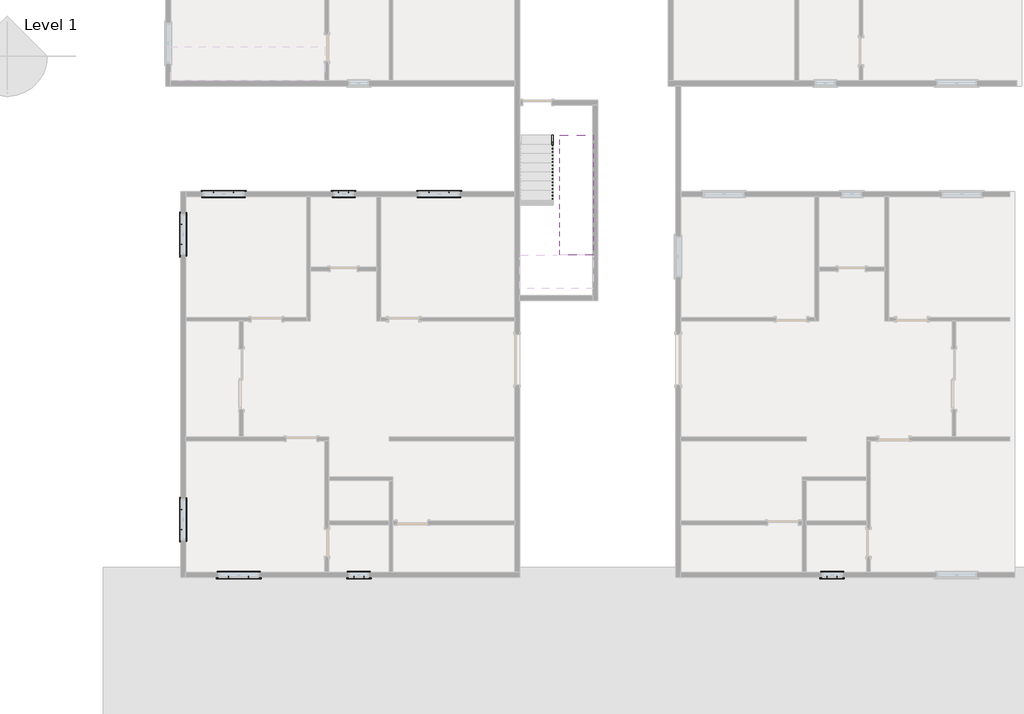
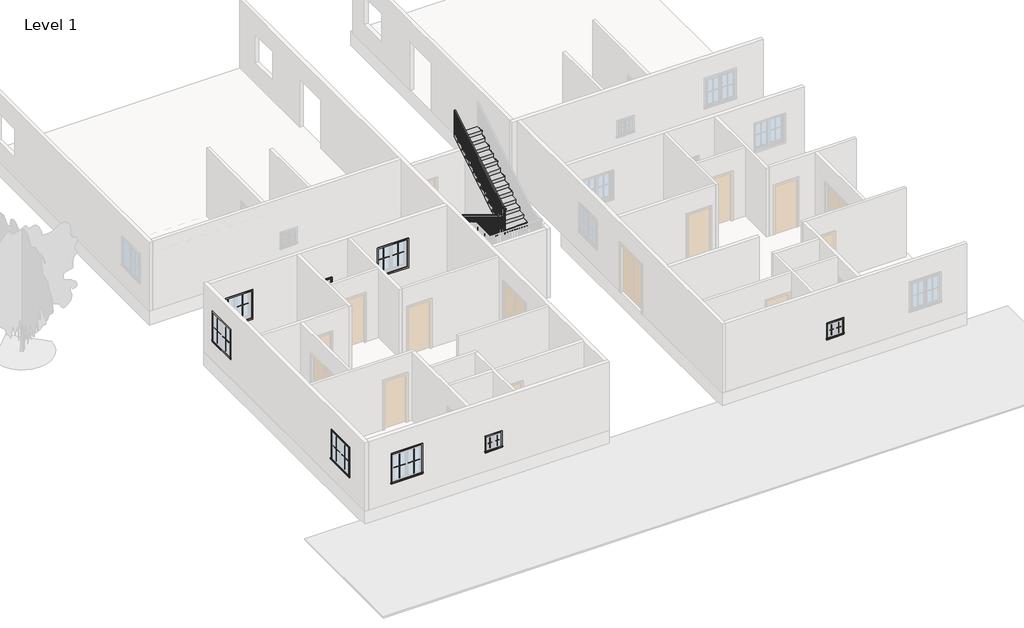
# One storey, part 5 of 7: 32 proxies, 1 railing, 1 stair flight.
"""IFC4 building model written with IfcOpenShell, lengths in millimetres."""

from ifc_helpers import new_model, si_unit, frame, origin, place, context, project, spatial, polyline, outline, extrude, faceted_brep, transform, mapped, element, save
from components import muntin_pattern_2x2_muntin_pattern_2x2_4dfeb3f3, muntin_pattern_2x2_muntin_pattern_2x2_e852a7e4, muntin_pattern_2x2_muntin_pattern_2x2_0961b91c, muntin_pattern_2x2_muntin_pattern_2x2_cae9449b, trim_window_exterior_flat_with_sill_7cfdd449, trim_window_exterior_flat_with_sill_858dc10d, trim_window_interior_flat_picture_frame_f1e0b15b, trim_window_interior_flat_picture_frame_3927330c

model = new_model("IFC4")

# Units and contexts
model_context = context("Model", 3, world=origin())
ifc_project = project(units=[si_unit("LENGTHUNIT", "METRE", prefix="MILLI")], contexts=[model_context])

# Site, building, storey
site = spatial("IfcSite", under=ifc_project)
building = spatial("IfcBuilding", under=site)
storey = spatial("IfcBuildingStorey", under=building, Name="Level 1", Elevation=0.0)

# Proxies
placement = place(None, origin())
muntin_pattern_2x2_muntin_pattern_2x2_shape = muntin_pattern_2x2_muntin_pattern_2x2_4dfeb3f3(model_context)
element("IfcBuildingElementProxy", 1, Name="Muntin Pattern_2x2 : Muntin Pattern_2x2", ObjectType="Muntin Pattern_2x2 : Muntin Pattern_2x2", at=placement, inside=storey, context=model_context, shape_type="MappedRepresentation", body=[
    mapped(muntin_pattern_2x2_muntin_pattern_2x2_shape, transform((-12764.9599256, -1071.5314015, 984.25), x_axis=(1.0, 0.0, 0.0), y_axis=(0.0, 1.0, 0.0), z_axis=(0.0, 0.0, 1.0))),
])
element("IfcBuildingElementProxy", 2, Name="Muntin Pattern_2x2 : Muntin Pattern_2x2", ObjectType="Muntin Pattern_2x2 : Muntin Pattern_2x2", at=placement, inside=storey, context=model_context, shape_type="MappedRepresentation", body=[
    mapped(muntin_pattern_2x2_muntin_pattern_2x2_shape, transform((-13747.0413899, -2660.6442701, 984.25), x_axis=(0.0, 1.0, 0.0), y_axis=(-1.0, 0.0, 0.0), z_axis=(0.0, 0.0, 1.0))),
])
element("IfcBuildingElementProxy", 3, Name="Muntin Pattern_2x2 : Muntin Pattern_2x2", ObjectType="Muntin Pattern_2x2 : Muntin Pattern_2x2", at=placement, inside=storey, context=model_context, shape_type="MappedRepresentation", body=[
    mapped(muntin_pattern_2x2_muntin_pattern_2x2_shape, transform((-6243.5099256, -1071.5314015, 984.25), x_axis=(1.0, 0.0, 0.0), y_axis=(0.0, 1.0, 0.0), z_axis=(0.0, 0.0, 1.0))),
])
element("IfcBuildingElementProxy", 4, Name="Muntin Pattern_2x2 : Muntin Pattern_2x2", ObjectType="Muntin Pattern_2x2 : Muntin Pattern_2x2", at=placement, inside=storey, context=model_context, shape_type="MappedRepresentation", body=[
    mapped(muntin_pattern_2x2_muntin_pattern_2x2_shape, transform((-13747.0413899, -11296.6442701, 984.25), x_axis=(0.0, 1.0, 0.0), y_axis=(-1.0, 0.0, 0.0), z_axis=(0.0, 0.0, 1.0))),
])
element("IfcBuildingElementProxy", 5, Name="Muntin Pattern_2x2 : Muntin Pattern_2x2", ObjectType="Muntin Pattern_2x2 : Muntin Pattern_2x2", at=placement, inside=storey, context=model_context, shape_type="MappedRepresentation", body=[
    mapped(muntin_pattern_2x2_muntin_pattern_2x2_shape, transform((-11701.3349256, -12736.4814015, 984.25), x_axis=(-1.0, 0.0, 0.0), y_axis=(0.0, -1.0, 0.0), z_axis=(0.0, 0.0, 1.0))),
])
muntin_pattern_2x2_muntin_pattern_2x2_2_shape = muntin_pattern_2x2_muntin_pattern_2x2_e852a7e4(model_context)
element("IfcBuildingElementProxy", 6, Name="Muntin Pattern_2x2 : Muntin Pattern_2x2", ObjectType="Muntin Pattern_2x2 : Muntin Pattern_2x2", at=placement, inside=storey, context=model_context, shape_type="MappedRepresentation", body=[
    mapped(muntin_pattern_2x2_muntin_pattern_2x2_2_shape, transform((-12158.5349256, -1071.5314015, 984.25), x_axis=(-1.0, 0.0, 0.0), y_axis=(0.0, -1.0, 0.0), z_axis=(0.0, 0.0, 1.0))),
])
element("IfcBuildingElementProxy", 7, Name="Muntin Pattern_2x2 : Muntin Pattern_2x2", ObjectType="Muntin Pattern_2x2 : Muntin Pattern_2x2", at=placement, inside=storey, context=model_context, shape_type="MappedRepresentation", body=[
    mapped(muntin_pattern_2x2_muntin_pattern_2x2_2_shape, transform((-13747.0413899, -2054.2192701, 984.25), x_axis=(0.0, -1.0, 0.0), y_axis=(1.0, 0.0, 0.0), z_axis=(0.0, 0.0, 1.0))),
])
element("IfcBuildingElementProxy", 8, Name="Muntin Pattern_2x2 : Muntin Pattern_2x2", ObjectType="Muntin Pattern_2x2 : Muntin Pattern_2x2", at=placement, inside=storey, context=model_context, shape_type="MappedRepresentation", body=[
    mapped(muntin_pattern_2x2_muntin_pattern_2x2_2_shape, transform((-5637.0849256, -1071.5314015, 984.25), x_axis=(-1.0, 0.0, 0.0), y_axis=(0.0, -1.0, 0.0), z_axis=(0.0, 0.0, 1.0))),
])
element("IfcBuildingElementProxy", 9, Name="Muntin Pattern_2x2 : Muntin Pattern_2x2", ObjectType="Muntin Pattern_2x2 : Muntin Pattern_2x2", at=placement, inside=storey, context=model_context, shape_type="MappedRepresentation", body=[
    mapped(muntin_pattern_2x2_muntin_pattern_2x2_2_shape, transform((-13747.0413899, -10690.2192701, 984.25), x_axis=(0.0, -1.0, 0.0), y_axis=(1.0, 0.0, 0.0), z_axis=(0.0, 0.0, 1.0))),
])
element("IfcBuildingElementProxy", 10, Name="Muntin Pattern_2x2 : Muntin Pattern_2x2", ObjectType="Muntin Pattern_2x2 : Muntin Pattern_2x2", at=placement, inside=storey, context=model_context, shape_type="MappedRepresentation", body=[
    mapped(muntin_pattern_2x2_muntin_pattern_2x2_2_shape, transform((-12307.7599256, -12736.4814015, 984.25), x_axis=(1.0, 0.0, 0.0), y_axis=(0.0, 1.0, 0.0), z_axis=(0.0, 0.0, 1.0))),
])
muntin_pattern_2x2_muntin_pattern_2x2_3_shape = muntin_pattern_2x2_muntin_pattern_2x2_0961b91c(model_context)
element("IfcBuildingElementProxy", 11, Name="Muntin Pattern_2x2 : Muntin Pattern_2x2", ObjectType="Muntin Pattern_2x2 : Muntin Pattern_2x2", at=placement, inside=storey, context=model_context, shape_type="MappedRepresentation", body=[
    mapped(muntin_pattern_2x2_muntin_pattern_2x2_3_shape, transform((-8980.3599256, -1071.5314015, 984.25), x_axis=(1.0, 0.0, 0.0), y_axis=(0.0, 1.0, 0.0), z_axis=(0.0, 0.0, 1.0))),
])
element("IfcBuildingElementProxy", 12, Name="Muntin Pattern_2x2 : Muntin Pattern_2x2", ObjectType="Muntin Pattern_2x2 : Muntin Pattern_2x2", at=placement, inside=storey, context=model_context, shape_type="MappedRepresentation", body=[
    mapped(muntin_pattern_2x2_muntin_pattern_2x2_3_shape, transform((-8216.4719485, -12736.4814015, 984.25), x_axis=(-1.0, 0.0, 0.0), y_axis=(0.0, -1.0, 0.0), z_axis=(0.0, 0.0, 1.0))),
])
element("IfcBuildingElementProxy", 13, Name="Muntin Pattern_2x2 : Muntin Pattern_2x2", ObjectType="Muntin Pattern_2x2 : Muntin Pattern_2x2", at=placement, inside=storey, context=model_context, shape_type="MappedRepresentation", body=[
    mapped(muntin_pattern_2x2_muntin_pattern_2x2_3_shape, transform((6102.7780515, -12736.4814015, 984.25), x_axis=(-1.0, 0.0, 0.0), y_axis=(0.0, -1.0, 0.0), z_axis=(0.0, 0.0, 1.0))),
])
muntin_pattern_2x2_muntin_pattern_2x2_4_shape = muntin_pattern_2x2_muntin_pattern_2x2_cae9449b(model_context)
element("IfcBuildingElementProxy", 14, Name="Muntin Pattern_2x2 : Muntin Pattern_2x2", ObjectType="Muntin Pattern_2x2 : Muntin Pattern_2x2", at=placement, inside=storey, context=model_context, shape_type="MappedRepresentation", body=[
    mapped(muntin_pattern_2x2_muntin_pattern_2x2_4_shape, transform((-8678.7349256, -1071.5314015, 984.25), x_axis=(-1.0, 0.0, 0.0), y_axis=(0.0, -1.0, 0.0), z_axis=(0.0, 0.0, 1.0))),
])
element("IfcBuildingElementProxy", 15, Name="Muntin Pattern_2x2 : Muntin Pattern_2x2", ObjectType="Muntin Pattern_2x2 : Muntin Pattern_2x2", at=placement, inside=storey, context=model_context, shape_type="MappedRepresentation", body=[
    mapped(muntin_pattern_2x2_muntin_pattern_2x2_4_shape, transform((-8518.0969485, -12736.4814015, 984.25), x_axis=(1.0, 0.0, 0.0), y_axis=(0.0, 1.0, 0.0), z_axis=(0.0, 0.0, 1.0))),
])
element("IfcBuildingElementProxy", 16, Name="Muntin Pattern_2x2 : Muntin Pattern_2x2", ObjectType="Muntin Pattern_2x2 : Muntin Pattern_2x2", at=placement, inside=storey, context=model_context, shape_type="MappedRepresentation", body=[
    mapped(muntin_pattern_2x2_muntin_pattern_2x2_4_shape, transform((5801.1530515, -12736.4814015, 984.25), x_axis=(1.0, 0.0, 0.0), y_axis=(0.0, 1.0, 0.0), z_axis=(0.0, 0.0, 1.0))),
])
trim_window_exterior_flat_with_sill_shape = trim_window_exterior_flat_with_sill_7cfdd449(model_context)
element("IfcBuildingElementProxy", 17, Name="Trim-Window-Exterior-Flat : with Sill", ObjectType="Trim-Window-Exterior-Flat : with Sill", at=placement, inside=storey, context=model_context, shape_type="MappedRepresentation", body=[
    mapped(trim_window_exterior_flat_with_sill_shape, transform((-12461.7474256, -1062.0064015, 2133.6), x_axis=(-1.0, 0.0, 0.0), y_axis=(0.0, 0.0, 1.0), z_axis=(0.0, 1.0, 0.0))),
])
element("IfcBuildingElementProxy", 18, Name="Trim-Window-Exterior-Flat : with Sill", ObjectType="Trim-Window-Exterior-Flat : with Sill", at=placement, inside=storey, context=model_context, shape_type="MappedRepresentation", body=[
    mapped(trim_window_exterior_flat_with_sill_shape, transform((-13756.5663899, -2357.4317701, 2133.6), x_axis=(0.0, -1.0, 0.0), y_axis=(0.0, 0.0, 1.0), z_axis=(-1.0, 0.0, 0.0))),
])
element("IfcBuildingElementProxy", 19, Name="Trim-Window-Exterior-Flat : with Sill", ObjectType="Trim-Window-Exterior-Flat : with Sill", at=placement, inside=storey, context=model_context, shape_type="MappedRepresentation", body=[
    mapped(trim_window_exterior_flat_with_sill_shape, transform((-5940.2974256, -1062.0064015, 2133.6), x_axis=(-1.0, 0.0, 0.0), y_axis=(0.0, 0.0, 1.0), z_axis=(0.0, 1.0, 0.0))),
])
element("IfcBuildingElementProxy", 20, Name="Trim-Window-Exterior-Flat : with Sill", ObjectType="Trim-Window-Exterior-Flat : with Sill", at=placement, inside=storey, context=model_context, shape_type="MappedRepresentation", body=[
    mapped(trim_window_exterior_flat_with_sill_shape, transform((-13756.5663899, -10993.4317701, 2133.6), x_axis=(0.0, -1.0, 0.0), y_axis=(0.0, 0.0, 1.0), z_axis=(-1.0, 0.0, 0.0))),
])
element("IfcBuildingElementProxy", 21, Name="Trim-Window-Exterior-Flat : with Sill", ObjectType="Trim-Window-Exterior-Flat : with Sill", at=placement, inside=storey, context=model_context, shape_type="MappedRepresentation", body=[
    mapped(trim_window_exterior_flat_with_sill_shape, transform((-12004.5474256, -12746.0064015, 2133.6), x_axis=(1.0, 0.0, 0.0), y_axis=(0.0, 0.0, 1.0), z_axis=(0.0, -1.0, 0.0))),
])
trim_window_exterior_flat_with_sill_2_shape = trim_window_exterior_flat_with_sill_858dc10d(model_context)
element("IfcBuildingElementProxy", 22, Name="Trim-Window-Exterior-Flat : with Sill", ObjectType="Trim-Window-Exterior-Flat : with Sill", at=placement, inside=storey, context=model_context, shape_type="MappedRepresentation", body=[
    mapped(trim_window_exterior_flat_with_sill_2_shape, transform((-8829.5474256, -1062.0064015, 1524.0), x_axis=(-1.0, 0.0, 0.0), y_axis=(0.0, 0.0, 1.0), z_axis=(0.0, 1.0, 0.0))),
])
element("IfcBuildingElementProxy", 23, Name="Trim-Window-Exterior-Flat : with Sill", ObjectType="Trim-Window-Exterior-Flat : with Sill", at=placement, inside=storey, context=model_context, shape_type="MappedRepresentation", body=[
    mapped(trim_window_exterior_flat_with_sill_2_shape, transform((-8367.2844485, -12746.0064015, 1524.0), x_axis=(1.0, 0.0, 0.0), y_axis=(0.0, 0.0, 1.0), z_axis=(0.0, -1.0, 0.0))),
])
element("IfcBuildingElementProxy", 24, Name="Trim-Window-Exterior-Flat : with Sill", ObjectType="Trim-Window-Exterior-Flat : with Sill", at=placement, inside=storey, context=model_context, shape_type="MappedRepresentation", body=[
    mapped(trim_window_exterior_flat_with_sill_2_shape, transform((5951.9655515, -12746.0064015, 1524.0), x_axis=(1.0, 0.0, 0.0), y_axis=(0.0, 0.0, 1.0), z_axis=(0.0, -1.0, 0.0))),
])
trim_window_interior_flat_picture_frame_shape = trim_window_interior_flat_picture_frame_f1e0b15b(model_context)
element("IfcBuildingElementProxy", 25, Name="Trim-Window-Interior-Flat : Picture Frame", ObjectType="Trim-Window-Interior-Flat : Picture Frame", at=placement, inside=storey, context=model_context, shape_type="MappedRepresentation", body=[
    mapped(trim_window_interior_flat_picture_frame_shape, transform((-12461.7474256, -1214.4064015, 2133.6), x_axis=(1.0, 0.0, 0.0), y_axis=(0.0, 0.0, 1.0), z_axis=(0.0, -1.0, 0.0))),
])
element("IfcBuildingElementProxy", 26, Name="Trim-Window-Interior-Flat : Picture Frame", ObjectType="Trim-Window-Interior-Flat : Picture Frame", at=placement, inside=storey, context=model_context, shape_type="MappedRepresentation", body=[
    mapped(trim_window_interior_flat_picture_frame_shape, transform((-13604.1663899, -2357.4317701, 2133.6), x_axis=(0.0, 1.0, 0.0), y_axis=(0.0, 0.0, 1.0), z_axis=(1.0, 0.0, 0.0))),
])
element("IfcBuildingElementProxy", 27, Name="Trim-Window-Interior-Flat : Picture Frame", ObjectType="Trim-Window-Interior-Flat : Picture Frame", at=placement, inside=storey, context=model_context, shape_type="MappedRepresentation", body=[
    mapped(trim_window_interior_flat_picture_frame_shape, transform((-5940.2974256, -1214.4064015, 2133.6), x_axis=(1.0, 0.0, 0.0), y_axis=(0.0, 0.0, 1.0), z_axis=(0.0, -1.0, 0.0))),
])
element("IfcBuildingElementProxy", 28, Name="Trim-Window-Interior-Flat : Picture Frame", ObjectType="Trim-Window-Interior-Flat : Picture Frame", at=placement, inside=storey, context=model_context, shape_type="MappedRepresentation", body=[
    mapped(trim_window_interior_flat_picture_frame_shape, transform((-13604.1663899, -10993.4317701, 2133.6), x_axis=(0.0, 1.0, 0.0), y_axis=(0.0, 0.0, 1.0), z_axis=(1.0, 0.0, 0.0))),
])
element("IfcBuildingElementProxy", 29, Name="Trim-Window-Interior-Flat : Picture Frame", ObjectType="Trim-Window-Interior-Flat : Picture Frame", at=placement, inside=storey, context=model_context, shape_type="MappedRepresentation", body=[
    mapped(trim_window_interior_flat_picture_frame_shape, transform((-12004.5474256, -12593.6064015, 2133.6), x_axis=(-1.0, 0.0, 0.0), y_axis=(0.0, 0.0, 1.0), z_axis=(0.0, 1.0, 0.0))),
])
trim_window_interior_flat_picture_frame_2_shape = trim_window_interior_flat_picture_frame_3927330c(model_context)
element("IfcBuildingElementProxy", 30, Name="Trim-Window-Interior-Flat : Picture Frame", ObjectType="Trim-Window-Interior-Flat : Picture Frame", at=placement, inside=storey, context=model_context, shape_type="MappedRepresentation", body=[
    mapped(trim_window_interior_flat_picture_frame_2_shape, transform((-8829.5474256, -1214.4064015, 1524.0), x_axis=(1.0, 0.0, 0.0), y_axis=(0.0, 0.0, 1.0), z_axis=(0.0, -1.0, 0.0))),
])
element("IfcBuildingElementProxy", 31, Name="Trim-Window-Interior-Flat : Picture Frame", ObjectType="Trim-Window-Interior-Flat : Picture Frame", at=placement, inside=storey, context=model_context, shape_type="MappedRepresentation", body=[
    mapped(trim_window_interior_flat_picture_frame_2_shape, transform((-8367.2844485, -12593.6064015, 1524.0), x_axis=(-1.0, 0.0, 0.0), y_axis=(0.0, 0.0, 1.0), z_axis=(0.0, 1.0, 0.0))),
])
element("IfcBuildingElementProxy", 32, Name="Trim-Window-Interior-Flat : Picture Frame", ObjectType="Trim-Window-Interior-Flat : Picture Frame", at=placement, inside=storey, context=model_context, shape_type="MappedRepresentation", body=[
    mapped(trim_window_interior_flat_picture_frame_2_shape, transform((5951.9655515, -12593.6064015, 1524.0), x_axis=(-1.0, 0.0, 0.0), y_axis=(0.0, 0.0, 1.0), z_axis=(0.0, 1.0, 0.0))),
])

# Railing
element("IfcRailing", 33, ObjectType="Handrail - Rectangular", at=placement, inside=storey, context=model_context, shape_type="SolidModel", body=[
    faceted_brep([(-2487.1844485, 646.3269271, 1083.7333333), (-2487.1844485, 646.3269271, 1024.3318731), (-2537.9844485, 646.3269271, 1024.3318731), (-2537.9844485, 646.3269271, 1083.7333333), (-2487.1844485, -2909.6730729, 3238.8848485), (-2487.1844485, -2960.4730729, 3210.271267), (-2537.9844485, -2960.4730729, 3210.271267), (-2537.9844485, -2909.6730729, 3238.8848485), (-2487.1844485, -2909.6730729, 3285.0666667), (-2487.1844485, -2960.4730729, 3234.2666667), (-2537.9844485, -2960.4730729, 3234.2666667), (-2537.9844485, -2909.6730729, 3285.0666667), (-2487.1844485, -2985.8730729, 3285.0666667), (-2487.1844485, -2985.8730729, 3234.2666667), (-2537.9844485, -3036.6730729, 3234.2666667), (-2537.9844485, -3036.6730729, 3285.0666667), (-2410.9844485, -2985.8730729, 3285.0666667), (-2410.9844485, -2985.8730729, 3234.2666667), (-2410.9844485, -3036.6730729, 3234.2666667), (-2410.9844485, -3036.6730729, 3285.0666667), (-2360.1844485, -2985.8730729, 3285.0666667), (-2309.3844485, -2985.8730729, 3234.2666667), (-2309.3844485, -3036.6730729, 3234.2666667), (-2360.1844485, -3036.6730729, 3285.0666667), (-2360.1844485, -2985.8730729, 3500.5818182), (-2309.3844485, -2985.8730729, 3449.7818182), (-2309.3844485, -3036.6730729, 3449.7818182), (-2360.1844485, -3036.6730729, 3500.5818182), (-2283.9844485, -2985.8730729, 3500.5818182), (-2283.9844485, -2985.8730729, 3449.7818182), (-2233.1844485, -3036.6730729, 3449.7818182), (-2233.1844485, -3036.6730729, 3500.5818182), (-2283.9844485, -2909.6730729, 3500.5818182), (-2283.9844485, -2895.4806634, 3449.7818182), (-2233.1844485, -2895.4806634, 3449.7818182), (-2233.1844485, -2909.6730729, 3500.5818182), (-2283.9844485, 646.3269271, 5655.7333333), (-2233.1844485, 646.3269271, 5655.7333333), (-2233.1844485, 646.3269271, 5596.3318731), (-2283.9844485, 646.3269271, 5596.3318731)], [[[0, 1, 2, 3]], [[1, 0, 4, 5]], [[2, 1, 5, 6]], [[3, 2, 6, 7]], [[0, 3, 7, 4]], [[5, 4, 8, 9]], [[6, 5, 9, 10]], [[7, 6, 10, 11]], [[4, 7, 11, 8]], [[9, 8, 12, 13]], [[10, 9, 13, 14]], [[11, 10, 14, 15]], [[8, 11, 15, 12]], [[13, 12, 16, 17]], [[14, 13, 17, 18]], [[15, 14, 18, 19]], [[12, 15, 19, 16]], [[17, 16, 20, 21]], [[18, 17, 21, 22]], [[19, 18, 22, 23]], [[16, 19, 23, 20]], [[21, 20, 24, 25]], [[22, 21, 25, 26]], [[23, 22, 26, 27]], [[20, 23, 27, 24]], [[25, 24, 28, 29]], [[26, 25, 29, 30]], [[27, 26, 30, 31]], [[24, 27, 31, 28]], [[29, 28, 32, 33]], [[30, 29, 33, 34]], [[31, 30, 34, 35]], [[28, 31, 35, 32]], [[36, 37, 38, 39]], [[33, 32, 36, 39]], [[34, 33, 39, 38]], [[35, 34, 38, 37]], [[32, 35, 37, 36]]]),
    extrude(outline(polyline([(554.2519271, 5540.5288428), (554.2519271, 4572.0), (535.2019271, 4572.0), (535.2019271, 5528.9833882), (554.2519271, 5540.5288428)])), frame((-2268.1094485, 0.0, 0.0), z_axis=(1.0, 0.0, 0.0), x_axis=(0.0, 1.0, 0.0)), (0.0, 0.0, 1.0), 19.05),
    extrude(outline(polyline([(452.6519271, 5478.9530852), (452.6519271, 4572.0), (433.6019271, 4572.0), (433.6019271, 5467.4076307), (452.6519271, 5478.9530852)])), frame((-2268.1094485, 0.0, 0.0), z_axis=(1.0, 0.0, 0.0), x_axis=(0.0, 1.0, 0.0)), (0.0, 0.0, 1.0), 19.05),
    extrude(outline(polyline([(351.0519271, 5417.3773276), (351.0519271, 4402.6666667), (332.0019271, 4402.6666667), (332.0019271, 5405.8318731), (351.0519271, 5417.3773276)])), frame((-2268.1094485, 0.0, 0.0), z_axis=(1.0, 0.0, 0.0), x_axis=(0.0, 1.0, 0.0)), (0.0, 0.0, 1.0), 19.05),
    extrude(outline(polyline([(249.4519271, 5355.80157), (249.4519271, 4402.6666667), (230.4019271, 4402.6666667), (230.4019271, 5344.2561155), (249.4519271, 5355.80157)])), frame((-2268.1094485, 0.0, 0.0), z_axis=(1.0, 0.0, 0.0), x_axis=(0.0, 1.0, 0.0)), (0.0, 0.0, 1.0), 19.05),
    extrude(outline(polyline([(147.8519271, 5294.2258125), (147.8519271, 4402.6666667), (128.8019271, 4402.6666667), (128.8019271, 5282.6803579), (147.8519271, 5294.2258125)])), frame((-2268.1094485, 0.0, 0.0), z_axis=(1.0, 0.0, 0.0), x_axis=(0.0, 1.0, 0.0)), (0.0, 0.0, 1.0), 19.05),
    extrude(outline(polyline([(46.2519271, 5232.6500549), (46.2519271, 4233.3333333), (27.2019271, 4233.3333333), (27.2019271, 5221.1046004), (46.2519271, 5232.6500549)])), frame((-2268.1094485, 0.0, 0.0), z_axis=(1.0, 0.0, 0.0), x_axis=(0.0, 1.0, 0.0)), (0.0, 0.0, 1.0), 19.05),
    extrude(outline(polyline([(-55.3480729, 5171.0742973), (-55.3480729, 4233.3333333), (-74.3980729, 4233.3333333), (-74.3980729, 5159.5288428), (-55.3480729, 5171.0742973)])), frame((-2268.1094485, 0.0, 0.0), z_axis=(1.0, 0.0, 0.0), x_axis=(0.0, 1.0, 0.0)), (0.0, 0.0, 1.0), 19.05),
    extrude(outline(polyline([(-156.9480729, 5109.4985397), (-156.9480729, 4233.3333333), (-175.9980729, 4233.3333333), (-175.9980729, 5097.9530852), (-156.9480729, 5109.4985397)])), frame((-2268.1094485, 0.0, 0.0), z_axis=(1.0, 0.0, 0.0), x_axis=(0.0, 1.0, 0.0)), (0.0, 0.0, 1.0), 19.05),
    extrude(outline(polyline([(-258.5480729, 5047.9227822), (-258.5480729, 4064.0), (-277.5980729, 4064.0), (-277.5980729, 5036.3773276), (-258.5480729, 5047.9227822)])), frame((-2268.1094485, 0.0, 0.0), z_axis=(1.0, 0.0, 0.0), x_axis=(0.0, 1.0, 0.0)), (0.0, 0.0, 1.0), 19.05),
    extrude(outline(polyline([(-360.1480729, 4986.3470246), (-360.1480729, 4064.0), (-379.1980729, 4064.0), (-379.1980729, 4974.80157), (-360.1480729, 4986.3470246)])), frame((-2268.1094485, 0.0, 0.0), z_axis=(1.0, 0.0, 0.0), x_axis=(0.0, 1.0, 0.0)), (0.0, 0.0, 1.0), 19.05),
    extrude(outline(polyline([(-461.7480729, 4924.771267), (-461.7480729, 4064.0), (-480.7980729, 4064.0), (-480.7980729, 4913.2258125), (-461.7480729, 4924.771267)])), frame((-2268.1094485, 0.0, 0.0), z_axis=(1.0, 0.0, 0.0), x_axis=(0.0, 1.0, 0.0)), (0.0, 0.0, 1.0), 19.05),
    extrude(outline(polyline([(-563.3480729, 4863.1955094), (-563.3480729, 3894.6666667), (-582.3980729, 3894.6666667), (-582.3980729, 4851.6500549), (-563.3480729, 4863.1955094)])), frame((-2268.1094485, 0.0, 0.0), z_axis=(1.0, 0.0, 0.0), x_axis=(0.0, 1.0, 0.0)), (0.0, 0.0, 1.0), 19.05),
    extrude(outline(polyline([(-664.9480729, 4801.6197519), (-664.9480729, 3894.6666667), (-683.9980729, 3894.6666667), (-683.9980729, 4790.0742973), (-664.9480729, 4801.6197519)])), frame((-2268.1094485, 0.0, 0.0), z_axis=(1.0, 0.0, 0.0), x_axis=(0.0, 1.0, 0.0)), (0.0, 0.0, 1.0), 19.05),
    extrude(outline(polyline([(-766.5480729, 4740.0439943), (-766.5480729, 3725.3333333), (-785.5980729, 3725.3333333), (-785.5980729, 4728.4985397), (-766.5480729, 4740.0439943)])), frame((-2268.1094485, 0.0, 0.0), z_axis=(1.0, 0.0, 0.0), x_axis=(0.0, 1.0, 0.0)), (0.0, 0.0, 1.0), 19.05),
    extrude(outline(polyline([(-868.1480729, 4678.4682367), (-868.1480729, 3725.3333333), (-887.1980729, 3725.3333333), (-887.1980729, 4666.9227822), (-868.1480729, 4678.4682367)])), frame((-2268.1094485, 0.0, 0.0), z_axis=(1.0, 0.0, 0.0), x_axis=(0.0, 1.0, 0.0)), (0.0, 0.0, 1.0), 19.05),
    extrude(outline(polyline([(-969.7480729, 4616.8924791), (-969.7480729, 3725.3333333), (-988.7980729, 3725.3333333), (-988.7980729, 4605.3470246), (-969.7480729, 4616.8924791)])), frame((-2268.1094485, 0.0, 0.0), z_axis=(1.0, 0.0, 0.0), x_axis=(0.0, 1.0, 0.0)), (0.0, 0.0, 1.0), 19.05),
    extrude(outline(polyline([(-1071.3480729, 4555.3167216), (-1071.3480729, 3556.0), (-1090.3980729, 3556.0), (-1090.3980729, 4543.771267), (-1071.3480729, 4555.3167216)])), frame((-2268.1094485, 0.0, 0.0), z_axis=(1.0, 0.0, 0.0), x_axis=(0.0, 1.0, 0.0)), (0.0, 0.0, 1.0), 19.05),
    extrude(outline(polyline([(-1172.9480729, 4493.740964), (-1172.9480729, 3556.0), (-1191.9980729, 3556.0), (-1191.9980729, 4482.1955094), (-1172.9480729, 4493.740964)])), frame((-2268.1094485, 0.0, 0.0), z_axis=(1.0, 0.0, 0.0), x_axis=(0.0, 1.0, 0.0)), (0.0, 0.0, 1.0), 19.05),
    extrude(outline(polyline([(-1274.5480729, 4432.1652064), (-1274.5480729, 3556.0), (-1293.5980729, 3556.0), (-1293.5980729, 4420.6197519), (-1274.5480729, 4432.1652064)])), frame((-2268.1094485, 0.0, 0.0), z_axis=(1.0, 0.0, 0.0), x_axis=(0.0, 1.0, 0.0)), (0.0, 0.0, 1.0), 19.05),
    extrude(outline(polyline([(-1376.1480729, 4370.5894488), (-1376.1480729, 3386.6666667), (-1395.1980729, 3386.6666667), (-1395.1980729, 4359.0439943), (-1376.1480729, 4370.5894488)])), frame((-2268.1094485, 0.0, 0.0), z_axis=(1.0, 0.0, 0.0), x_axis=(0.0, 1.0, 0.0)), (0.0, 0.0, 1.0), 19.05),
    extrude(outline(polyline([(-1477.7480729, 4309.0136913), (-1477.7480729, 3386.6666667), (-1496.7980729, 3386.6666667), (-1496.7980729, 4297.4682367), (-1477.7480729, 4309.0136913)])), frame((-2268.1094485, 0.0, 0.0), z_axis=(1.0, 0.0, 0.0), x_axis=(0.0, 1.0, 0.0)), (0.0, 0.0, 1.0), 19.05),
    extrude(outline(polyline([(-1579.3480729, 4247.4379337), (-1579.3480729, 3386.6666667), (-1598.3980729, 3386.6666667), (-1598.3980729, 4235.8924791), (-1579.3480729, 4247.4379337)])), frame((-2268.1094485, 0.0, 0.0), z_axis=(1.0, 0.0, 0.0), x_axis=(0.0, 1.0, 0.0)), (0.0, 0.0, 1.0), 19.05),
    extrude(outline(polyline([(-1680.9480729, 4185.8621761), (-1680.9480729, 3217.3333333), (-1699.9980729, 3217.3333333), (-1699.9980729, 4174.3167216), (-1680.9480729, 4185.8621761)])), frame((-2268.1094485, 0.0, 0.0), z_axis=(1.0, 0.0, 0.0), x_axis=(0.0, 1.0, 0.0)), (0.0, 0.0, 1.0), 19.05),
    extrude(outline(polyline([(-1782.5480729, 4124.2864185), (-1782.5480729, 3217.3333333), (-1801.5980729, 3217.3333333), (-1801.5980729, 4112.740964), (-1782.5480729, 4124.2864185)])), frame((-2268.1094485, 0.0, 0.0), z_axis=(1.0, 0.0, 0.0), x_axis=(0.0, 1.0, 0.0)), (0.0, 0.0, 1.0), 19.05),
    extrude(outline(polyline([(-1884.1480729, 4062.710661), (-1884.1480729, 3048.0), (-1903.1980729, 3048.0), (-1903.1980729, 4051.1652064), (-1884.1480729, 4062.710661)])), frame((-2268.1094485, 0.0, 0.0), z_axis=(1.0, 0.0, 0.0), x_axis=(0.0, 1.0, 0.0)), (0.0, 0.0, 1.0), 19.05),
    extrude(outline(polyline([(-1985.7480729, 4001.1349034), (-1985.7480729, 3048.0), (-2004.7980729, 3048.0), (-2004.7980729, 3989.5894488), (-1985.7480729, 4001.1349034)])), frame((-2268.1094485, 0.0, 0.0), z_axis=(1.0, 0.0, 0.0), x_axis=(0.0, 1.0, 0.0)), (0.0, 0.0, 1.0), 19.05),
    extrude(outline(polyline([(-2087.3480729, 3939.5591458), (-2087.3480729, 3048.0), (-2106.3980729, 3048.0), (-2106.3980729, 3928.0136913), (-2087.3480729, 3939.5591458)])), frame((-2268.1094485, 0.0, 0.0), z_axis=(1.0, 0.0, 0.0), x_axis=(0.0, 1.0, 0.0)), (0.0, 0.0, 1.0), 19.05),
    extrude(outline(polyline([(-2188.9480729, 3877.9833882), (-2188.9480729, 2878.6666667), (-2207.9980729, 2878.6666667), (-2207.9980729, 3866.4379337), (-2188.9480729, 3877.9833882)])), frame((-2268.1094485, 0.0, 0.0), z_axis=(1.0, 0.0, 0.0), x_axis=(0.0, 1.0, 0.0)), (0.0, 0.0, 1.0), 19.05),
    extrude(outline(polyline([(-2290.5480729, 3816.4076307), (-2290.5480729, 2878.6666667), (-2309.5980729, 2878.6666667), (-2309.5980729, 3804.8621761), (-2290.5480729, 3816.4076307)])), frame((-2268.1094485, 0.0, 0.0), z_axis=(1.0, 0.0, 0.0), x_axis=(0.0, 1.0, 0.0)), (0.0, 0.0, 1.0), 19.05),
    extrude(outline(polyline([(-2392.1480729, 3754.8318731), (-2392.1480729, 2878.6666667), (-2411.1980729, 2878.6666667), (-2411.1980729, 3743.2864185), (-2392.1480729, 3754.8318731)])), frame((-2268.1094485, 0.0, 0.0), z_axis=(1.0, 0.0, 0.0), x_axis=(0.0, 1.0, 0.0)), (0.0, 0.0, 1.0), 19.05),
    extrude(outline(polyline([(-2493.7480729, 3693.2561155), (-2493.7480729, 2709.3333333), (-2512.7980729, 2709.3333333), (-2512.7980729, 3681.710661), (-2493.7480729, 3693.2561155)])), frame((-2268.1094485, 0.0, 0.0), z_axis=(1.0, 0.0, 0.0), x_axis=(0.0, 1.0, 0.0)), (0.0, 0.0, 1.0), 19.05),
    extrude(outline(polyline([(-2595.3480729, 3631.6803579), (-2595.3480729, 2709.3333333), (-2614.3980729, 2709.3333333), (-2614.3980729, 3620.1349034), (-2595.3480729, 3631.6803579)])), frame((-2268.1094485, 0.0, 0.0), z_axis=(1.0, 0.0, 0.0), x_axis=(0.0, 1.0, 0.0)), (0.0, 0.0, 1.0), 19.05),
    extrude(outline(polyline([(-2696.9480729, 3570.1046004), (-2696.9480729, 2709.3333333), (-2715.9980729, 2709.3333333), (-2715.9980729, 3558.5591458), (-2696.9480729, 3570.1046004)])), frame((-2268.1094485, 0.0, 0.0), z_axis=(1.0, 0.0, 0.0), x_axis=(0.0, 1.0, 0.0)), (0.0, 0.0, 1.0), 19.05),
    extrude(outline(polyline([(-2798.5480729, 3508.5288428), (-2798.5480729, 2540.0), (-2817.5980729, 2540.0), (-2817.5980729, 3496.9833882), (-2798.5480729, 3508.5288428)])), frame((-2268.1094485, 0.0, 0.0), z_axis=(1.0, 0.0, 0.0), x_axis=(0.0, 1.0, 0.0)), (0.0, 0.0, 1.0), 19.05),
    extrude(outline(polyline([(-2900.1480729, 3446.9530852), (-2900.1480729, 2540.0), (-2919.1980729, 2540.0), (-2919.1980729, 3435.4076307), (-2900.1480729, 3446.9530852)])), frame((-2268.1094485, 0.0, 0.0), z_axis=(1.0, 0.0, 0.0), x_axis=(0.0, 1.0, 0.0)), (0.0, 0.0, 1.0), 19.05),
    extrude(outline(polyline([(-2318.9094485, -3001.7480729), (-2299.8594485, -3001.7480729), (-2299.8594485, -3020.7980729), (-2318.9094485, -3020.7980729), (-2318.9094485, -3001.7480729)])), frame((0.0, 0.0, 2370.6666667), z_axis=(0.0, 0.0, 1.0), x_axis=(1.0, 0.0, 0.0)), (0.0, 0.0, 1.0), 1079.1151515),
    extrude(outline(polyline([(-2420.5094485, -3001.7480729), (-2401.4594485, -3001.7480729), (-2401.4594485, -3020.7980729), (-2420.5094485, -3020.7980729), (-2420.5094485, -3001.7480729)])), frame((0.0, 0.0, 2370.6666667), z_axis=(0.0, 0.0, 1.0), x_axis=(1.0, 0.0, 0.0)), (0.0, 0.0, 1.0), 863.6),
    extrude(outline(polyline([(-2900.1480729, 3173.710661), (-2900.1480729, 2201.3333333), (-2919.1980729, 2201.3333333), (-2919.1980729, 3185.2561155), (-2900.1480729, 3173.710661)])), frame((-2522.1094485, 0.0, 0.0), z_axis=(1.0, 0.0, 0.0), x_axis=(0.0, 1.0, 0.0)), (0.0, 0.0, 1.0), 19.05),
    extrude(outline(polyline([(-2798.5480729, 3112.1349034), (-2798.5480729, 2201.3333333), (-2817.5980729, 2201.3333333), (-2817.5980729, 3123.6803579), (-2798.5480729, 3112.1349034)])), frame((-2522.1094485, 0.0, 0.0), z_axis=(1.0, 0.0, 0.0), x_axis=(0.0, 1.0, 0.0)), (0.0, 0.0, 1.0), 19.05),
    extrude(outline(polyline([(-2696.9480729, 3050.5591458), (-2696.9480729, 2201.3333333), (-2715.9980729, 2201.3333333), (-2715.9980729, 3062.1046004), (-2696.9480729, 3050.5591458)])), frame((-2522.1094485, 0.0, 0.0), z_axis=(1.0, 0.0, 0.0), x_axis=(0.0, 1.0, 0.0)), (0.0, 0.0, 1.0), 19.05),
    extrude(outline(polyline([(-2595.3480729, 2988.9833882), (-2595.3480729, 2032.0), (-2614.3980729, 2032.0), (-2614.3980729, 3000.5288428), (-2595.3480729, 2988.9833882)])), frame((-2522.1094485, 0.0, 0.0), z_axis=(1.0, 0.0, 0.0), x_axis=(0.0, 1.0, 0.0)), (0.0, 0.0, 1.0), 19.05),
    extrude(outline(polyline([(-2493.7480729, 2927.4076307), (-2493.7480729, 2032.0), (-2512.7980729, 2032.0), (-2512.7980729, 2938.9530852), (-2493.7480729, 2927.4076307)])), frame((-2522.1094485, 0.0, 0.0), z_axis=(1.0, 0.0, 0.0), x_axis=(0.0, 1.0, 0.0)), (0.0, 0.0, 1.0), 19.05),
    extrude(outline(polyline([(-2392.1480729, 2865.8318731), (-2392.1480729, 1862.6666667), (-2411.1980729, 1862.6666667), (-2411.1980729, 2877.3773276), (-2392.1480729, 2865.8318731)])), frame((-2522.1094485, 0.0, 0.0), z_axis=(1.0, 0.0, 0.0), x_axis=(0.0, 1.0, 0.0)), (0.0, 0.0, 1.0), 19.05),
    extrude(outline(polyline([(-2290.5480729, 2804.2561155), (-2290.5480729, 1862.6666667), (-2309.5980729, 1862.6666667), (-2309.5980729, 2815.80157), (-2290.5480729, 2804.2561155)])), frame((-2522.1094485, 0.0, 0.0), z_axis=(1.0, 0.0, 0.0), x_axis=(0.0, 1.0, 0.0)), (0.0, 0.0, 1.0), 19.05),
    extrude(outline(polyline([(-2188.9480729, 2742.6803579), (-2188.9480729, 1862.6666667), (-2207.9980729, 1862.6666667), (-2207.9980729, 2754.2258125), (-2188.9480729, 2742.6803579)])), frame((-2522.1094485, 0.0, 0.0), z_axis=(1.0, 0.0, 0.0), x_axis=(0.0, 1.0, 0.0)), (0.0, 0.0, 1.0), 19.05),
    extrude(outline(polyline([(-2087.3480729, 2681.1046004), (-2087.3480729, 1693.3333333), (-2106.3980729, 1693.3333333), (-2106.3980729, 2692.6500549), (-2087.3480729, 2681.1046004)])), frame((-2522.1094485, 0.0, 0.0), z_axis=(1.0, 0.0, 0.0), x_axis=(0.0, 1.0, 0.0)), (0.0, 0.0, 1.0), 19.05),
    extrude(outline(polyline([(-1985.7480729, 2619.5288428), (-1985.7480729, 1693.3333333), (-2004.7980729, 1693.3333333), (-2004.7980729, 2631.0742973), (-1985.7480729, 2619.5288428)])), frame((-2522.1094485, 0.0, 0.0), z_axis=(1.0, 0.0, 0.0), x_axis=(0.0, 1.0, 0.0)), (0.0, 0.0, 1.0), 19.05),
    extrude(outline(polyline([(-1884.1480729, 2557.9530852), (-1884.1480729, 1693.3333333), (-1903.1980729, 1693.3333333), (-1903.1980729, 2569.4985397), (-1884.1480729, 2557.9530852)])), frame((-2522.1094485, 0.0, 0.0), z_axis=(1.0, 0.0, 0.0), x_axis=(0.0, 1.0, 0.0)), (0.0, 0.0, 1.0), 19.05),
    extrude(outline(polyline([(-1782.5480729, 2496.3773276), (-1782.5480729, 1524.0), (-1801.5980729, 1524.0), (-1801.5980729, 2507.9227822), (-1782.5480729, 2496.3773276)])), frame((-2522.1094485, 0.0, 0.0), z_axis=(1.0, 0.0, 0.0), x_axis=(0.0, 1.0, 0.0)), (0.0, 0.0, 1.0), 19.05),
    extrude(outline(polyline([(-1680.9480729, 2434.80157), (-1680.9480729, 1524.0), (-1699.9980729, 1524.0), (-1699.9980729, 2446.3470246), (-1680.9480729, 2434.80157)])), frame((-2522.1094485, 0.0, 0.0), z_axis=(1.0, 0.0, 0.0), x_axis=(0.0, 1.0, 0.0)), (0.0, 0.0, 1.0), 19.05),
    extrude(outline(polyline([(-1579.3480729, 2373.2258125), (-1579.3480729, 1524.0), (-1598.3980729, 1524.0), (-1598.3980729, 2384.771267), (-1579.3480729, 2373.2258125)])), frame((-2522.1094485, 0.0, 0.0), z_axis=(1.0, 0.0, 0.0), x_axis=(0.0, 1.0, 0.0)), (0.0, 0.0, 1.0), 19.05),
    extrude(outline(polyline([(-1477.7480729, 2311.6500549), (-1477.7480729, 1354.6666667), (-1496.7980729, 1354.6666667), (-1496.7980729, 2323.1955094), (-1477.7480729, 2311.6500549)])), frame((-2522.1094485, 0.0, 0.0), z_axis=(1.0, 0.0, 0.0), x_axis=(0.0, 1.0, 0.0)), (0.0, 0.0, 1.0), 19.05),
    extrude(outline(polyline([(-1376.1480729, 2250.0742973), (-1376.1480729, 1354.6666667), (-1395.1980729, 1354.6666667), (-1395.1980729, 2261.6197519), (-1376.1480729, 2250.0742973)])), frame((-2522.1094485, 0.0, 0.0), z_axis=(1.0, 0.0, 0.0), x_axis=(0.0, 1.0, 0.0)), (0.0, 0.0, 1.0), 19.05),
    extrude(outline(polyline([(-1274.5480729, 2188.4985397), (-1274.5480729, 1185.3333333), (-1293.5980729, 1185.3333333), (-1293.5980729, 2200.0439943), (-1274.5480729, 2188.4985397)])), frame((-2522.1094485, 0.0, 0.0), z_axis=(1.0, 0.0, 0.0), x_axis=(0.0, 1.0, 0.0)), (0.0, 0.0, 1.0), 19.05),
    extrude(outline(polyline([(-1172.9480729, 2126.9227822), (-1172.9480729, 1185.3333333), (-1191.9980729, 1185.3333333), (-1191.9980729, 2138.4682367), (-1172.9480729, 2126.9227822)])), frame((-2522.1094485, 0.0, 0.0), z_axis=(1.0, 0.0, 0.0), x_axis=(0.0, 1.0, 0.0)), (0.0, 0.0, 1.0), 19.05),
    extrude(outline(polyline([(-1071.3480729, 2065.3470246), (-1071.3480729, 1185.3333333), (-1090.3980729, 1185.3333333), (-1090.3980729, 2076.8924791), (-1071.3480729, 2065.3470246)])), frame((-2522.1094485, 0.0, 0.0), z_axis=(1.0, 0.0, 0.0), x_axis=(0.0, 1.0, 0.0)), (0.0, 0.0, 1.0), 19.05),
    extrude(outline(polyline([(-969.7480729, 2003.771267), (-969.7480729, 1016.0), (-988.7980729, 1016.0), (-988.7980729, 2015.3167216), (-969.7480729, 2003.771267)])), frame((-2522.1094485, 0.0, 0.0), z_axis=(1.0, 0.0, 0.0), x_axis=(0.0, 1.0, 0.0)), (0.0, 0.0, 1.0), 19.05),
    extrude(outline(polyline([(-868.1480729, 1942.1955094), (-868.1480729, 1016.0), (-887.1980729, 1016.0), (-887.1980729, 1953.740964), (-868.1480729, 1942.1955094)])), frame((-2522.1094485, 0.0, 0.0), z_axis=(1.0, 0.0, 0.0), x_axis=(0.0, 1.0, 0.0)), (0.0, 0.0, 1.0), 19.05),
    extrude(outline(polyline([(-766.5480729, 1880.6197519), (-766.5480729, 1016.0), (-785.5980729, 1016.0), (-785.5980729, 1892.1652064), (-766.5480729, 1880.6197519)])), frame((-2522.1094485, 0.0, 0.0), z_axis=(1.0, 0.0, 0.0), x_axis=(0.0, 1.0, 0.0)), (0.0, 0.0, 1.0), 19.05),
    extrude(outline(polyline([(-664.9480729, 1819.0439943), (-664.9480729, 846.6666667), (-683.9980729, 846.6666667), (-683.9980729, 1830.5894488), (-664.9480729, 1819.0439943)])), frame((-2522.1094485, 0.0, 0.0), z_axis=(1.0, 0.0, 0.0), x_axis=(0.0, 1.0, 0.0)), (0.0, 0.0, 1.0), 19.05),
    extrude(outline(polyline([(-563.3480729, 1757.4682367), (-563.3480729, 846.6666667), (-582.3980729, 846.6666667), (-582.3980729, 1769.0136913), (-563.3480729, 1757.4682367)])), frame((-2522.1094485, 0.0, 0.0), z_axis=(1.0, 0.0, 0.0), x_axis=(0.0, 1.0, 0.0)), (0.0, 0.0, 1.0), 19.05),
    extrude(outline(polyline([(-461.7480729, 1695.8924791), (-461.7480729, 846.6666667), (-480.7980729, 846.6666667), (-480.7980729, 1707.4379337), (-461.7480729, 1695.8924791)])), frame((-2522.1094485, 0.0, 0.0), z_axis=(1.0, 0.0, 0.0), x_axis=(0.0, 1.0, 0.0)), (0.0, 0.0, 1.0), 19.05),
    extrude(outline(polyline([(-360.1480729, 1634.3167216), (-360.1480729, 677.3333333), (-379.1980729, 677.3333333), (-379.1980729, 1645.8621761), (-360.1480729, 1634.3167216)])), frame((-2522.1094485, 0.0, 0.0), z_axis=(1.0, 0.0, 0.0), x_axis=(0.0, 1.0, 0.0)), (0.0, 0.0, 1.0), 19.05),
    extrude(outline(polyline([(-258.5480729, 1572.740964), (-258.5480729, 677.3333333), (-277.5980729, 677.3333333), (-277.5980729, 1584.2864185), (-258.5480729, 1572.740964)])), frame((-2522.1094485, 0.0, 0.0), z_axis=(1.0, 0.0, 0.0), x_axis=(0.0, 1.0, 0.0)), (0.0, 0.0, 1.0), 19.05),
    extrude(outline(polyline([(-156.9480729, 1511.1652064), (-156.9480729, 508.0), (-175.9980729, 508.0), (-175.9980729, 1522.710661), (-156.9480729, 1511.1652064)])), frame((-2522.1094485, 0.0, 0.0), z_axis=(1.0, 0.0, 0.0), x_axis=(0.0, 1.0, 0.0)), (0.0, 0.0, 1.0), 19.05),
    extrude(outline(polyline([(-55.3480729, 1449.5894488), (-55.3480729, 508.0), (-74.3980729, 508.0), (-74.3980729, 1461.1349034), (-55.3480729, 1449.5894488)])), frame((-2522.1094485, 0.0, 0.0), z_axis=(1.0, 0.0, 0.0), x_axis=(0.0, 1.0, 0.0)), (0.0, 0.0, 1.0), 19.05),
    extrude(outline(polyline([(46.2519271, 1388.0136913), (46.2519271, 508.0), (27.2019271, 508.0), (27.2019271, 1399.5591458), (46.2519271, 1388.0136913)])), frame((-2522.1094485, 0.0, 0.0), z_axis=(1.0, 0.0, 0.0), x_axis=(0.0, 1.0, 0.0)), (0.0, 0.0, 1.0), 19.05),
    extrude(outline(polyline([(147.8519271, 1326.4379337), (147.8519271, 338.6666667), (128.8019271, 338.6666667), (128.8019271, 1337.9833882), (147.8519271, 1326.4379337)])), frame((-2522.1094485, 0.0, 0.0), z_axis=(1.0, 0.0, 0.0), x_axis=(0.0, 1.0, 0.0)), (0.0, 0.0, 1.0), 19.05),
    extrude(outline(polyline([(249.4519271, 1264.8621761), (249.4519271, 338.6666667), (230.4019271, 338.6666667), (230.4019271, 1276.4076307), (249.4519271, 1264.8621761)])), frame((-2522.1094485, 0.0, 0.0), z_axis=(1.0, 0.0, 0.0), x_axis=(0.0, 1.0, 0.0)), (0.0, 0.0, 1.0), 19.05),
    extrude(outline(polyline([(351.0519271, 1203.2864185), (351.0519271, 338.6666667), (332.0019271, 338.6666667), (332.0019271, 1214.8318731), (351.0519271, 1203.2864185)])), frame((-2522.1094485, 0.0, 0.0), z_axis=(1.0, 0.0, 0.0), x_axis=(0.0, 1.0, 0.0)), (0.0, 0.0, 1.0), 19.05),
    extrude(outline(polyline([(452.6519271, 1141.710661), (452.6519271, 169.3333333), (433.6019271, 169.3333333), (433.6019271, 1153.2561155), (452.6519271, 1141.710661)])), frame((-2522.1094485, 0.0, 0.0), z_axis=(1.0, 0.0, 0.0), x_axis=(0.0, 1.0, 0.0)), (0.0, 0.0, 1.0), 19.05),
    extrude(outline(polyline([(554.2519271, 1080.1349034), (554.2519271, 169.3333333), (535.2019271, 169.3333333), (535.2019271, 1091.6803579), (554.2519271, 1080.1349034)])), frame((-2522.1094485, 0.0, 0.0), z_axis=(1.0, 0.0, 0.0), x_axis=(0.0, 1.0, 0.0)), (0.0, 0.0, 1.0), 19.05),
    extrude(outline(polyline([(-2268.1094485, -3001.7480729), (-2249.0594485, -3001.7480729), (-2249.0594485, -3020.7980729), (-2268.1094485, -3020.7980729), (-2268.1094485, -3001.7480729)])), frame((0.0, 0.0, 2370.6666667), z_axis=(0.0, 0.0, 1.0), x_axis=(1.0, 0.0, 0.0)), (0.0, 0.0, 1.0), 1079.1151515),
    extrude(outline(polyline([(-2503.0594485, -3001.7480729), (-2503.0594485, -3020.7980729), (-2522.1094485, -3020.7980729), (-2522.1094485, -3001.7480729), (-2503.0594485, -3001.7480729)])), frame((0.0, 0.0, 2370.6666667), z_axis=(0.0, 0.0, 1.0), x_axis=(1.0, 0.0, 0.0)), (0.0, 0.0, 1.0), 863.6),
    extrude(outline(polyline([(646.3269271, 5596.3318731), (646.3269271, 4572.0), (627.2769271, 4572.0), (627.2769271, 5584.7864185), (646.3269271, 5596.3318731)])), frame((-2268.1094485, 0.0, 0.0), z_axis=(1.0, 0.0, 0.0), x_axis=(0.0, 1.0, 0.0)), (0.0, 0.0, 1.0), 19.05),
    extrude(outline(polyline([(646.3269271, 1024.3318731), (646.3269271, 169.3333333), (627.2769271, 169.3333333), (627.2769271, 1035.8773276), (646.3269271, 1024.3318731)])), frame((-2522.1094485, 0.0, 0.0), z_axis=(1.0, 0.0, 0.0), x_axis=(0.0, 1.0, 0.0)), (0.0, 0.0, 1.0), 19.05),
])

# Stair flight
element("IfcStairFlight", 34, ObjectType="3/4\" Nosing", at=placement, inside=storey, context=model_context, shape_type="Brep", body=[
    faceted_brep([(-2283.9844485, -2985.8730729, 2540.0), (-1267.9844485, -2985.8730729, 2540.0), (-1267.9844485, -2687.4230729, 2540.0), (-2283.9844485, -2687.4230729, 2540.0), (-2283.9844485, -2687.4230729, 2465.7481747), (-2283.9844485, -2966.8230729, 2296.4148413), (-2283.9844485, -2966.8230729, 2370.6666667), (-1267.9844485, -2966.8230729, 2370.6666667), (-1267.9844485, -2966.8230729, 2296.4148413), (-1267.9844485, -2687.4230729, 2465.7481747), (-2283.9844485, -2706.4730729, 2709.3333333), (-1267.9844485, -2706.4730729, 2709.3333333), (-1267.9844485, -2408.0230729, 2709.3333333), (-2283.9844485, -2408.0230729, 2709.3333333), (-2283.9844485, -2408.0230729, 2635.081508), (-1267.9844485, -2408.0230729, 2635.081508), (-2283.9844485, -2427.0730729, 2878.6666667), (-1267.9844485, -2427.0730729, 2878.6666667), (-1267.9844485, -2128.6230729, 2878.6666667), (-2283.9844485, -2128.6230729, 2878.6666667), (-2283.9844485, -2128.6230729, 2804.4148413), (-1267.9844485, -2128.6230729, 2804.4148413), (-2283.9844485, -2147.6730729, 3048.0), (-1267.9844485, -2147.6730729, 3048.0), (-1267.9844485, -1849.2230729, 3048.0), (-2283.9844485, -1849.2230729, 3048.0), (-2283.9844485, -1849.2230729, 2973.7481747), (-1267.9844485, -1849.2230729, 2973.7481747), (-2283.9844485, -1868.2730729, 3217.3333333), (-1267.9844485, -1868.2730729, 3217.3333333), (-1267.9844485, -1569.8230729, 3217.3333333), (-2283.9844485, -1569.8230729, 3217.3333333), (-2283.9844485, -1569.8230729, 3143.081508), (-1267.9844485, -1569.8230729, 3143.081508), (-2283.9844485, -1588.8730729, 3386.6666667), (-1267.9844485, -1588.8730729, 3386.6666667), (-1267.9844485, -1290.4230729, 3386.6666667), (-2283.9844485, -1290.4230729, 3386.6666667), (-2283.9844485, -1290.4230729, 3312.4148413), (-1267.9844485, -1290.4230729, 3312.4148413), (-2283.9844485, -1309.4730729, 3556.0), (-1267.9844485, -1309.4730729, 3556.0), (-1267.9844485, -1011.0230729, 3556.0), (-2283.9844485, -1011.0230729, 3556.0), (-2283.9844485, -1011.0230729, 3481.7481747), (-1267.9844485, -1011.0230729, 3481.7481747), (-2283.9844485, -1030.0730729, 3725.3333333), (-1267.9844485, -1030.0730729, 3725.3333333), (-1267.9844485, -731.6230729, 3725.3333333), (-2283.9844485, -731.6230729, 3725.3333333), (-2283.9844485, -731.6230729, 3651.081508), (-1267.9844485, -731.6230729, 3651.081508), (-2283.9844485, -750.6730729, 3894.6666667), (-1267.9844485, -750.6730729, 3894.6666667), (-1267.9844485, -452.2230729, 3894.6666667), (-2283.9844485, -452.2230729, 3894.6666667), (-2283.9844485, -452.2230729, 3820.4148413), (-1267.9844485, -452.2230729, 3820.4148413), (-2283.9844485, -471.2730729, 4064.0), (-1267.9844485, -471.2730729, 4064.0), (-1267.9844485, -172.8230729, 4064.0), (-2283.9844485, -172.8230729, 4064.0), (-2283.9844485, -172.8230729, 3989.7481747), (-1267.9844485, -172.8230729, 3989.7481747), (-2283.9844485, -191.8730729, 4233.3333333), (-1267.9844485, -191.8730729, 4233.3333333), (-1267.9844485, 106.5769271, 4233.3333333), (-2283.9844485, 106.5769271, 4233.3333333), (-2283.9844485, 106.5769271, 4159.081508), (-1267.9844485, 106.5769271, 4159.081508), (-2283.9844485, 87.5269271, 4402.6666667), (-1267.9844485, 87.5269271, 4402.6666667), (-1267.9844485, 385.9769271, 4402.6666667), (-2283.9844485, 385.9769271, 4402.6666667), (-2283.9844485, 385.9769271, 4328.4148413), (-1267.9844485, 385.9769271, 4328.4148413), (-2283.9844485, 366.9269271, 4572.0), (-1267.9844485, 366.9269271, 4572.0), (-1267.9844485, 646.3269271, 4572.0), (-2283.9844485, 646.3269271, 4572.0), (-2283.9844485, 646.3269271, 4486.2027201), (-1267.9844485, 646.3269271, 4486.2027201)], [[[0, 1, 2, 3]], [[0, 3, 4, 5, 6]], [[7, 6, 5, 8]], [[2, 1, 7, 8, 9]], [[10, 11, 12, 13]], [[10, 13, 14, 4, 3]], [[12, 11, 2, 9, 15]], [[16, 17, 18, 19]], [[16, 19, 20, 14, 13]], [[18, 17, 12, 15, 21]], [[22, 23, 24, 25]], [[22, 25, 26, 20, 19]], [[24, 23, 18, 21, 27]], [[28, 29, 30, 31]], [[28, 31, 32, 26, 25]], [[30, 29, 24, 27, 33]], [[34, 35, 36, 37]], [[34, 37, 38, 32, 31]], [[36, 35, 30, 33, 39]], [[40, 41, 42, 43]], [[40, 43, 44, 38, 37]], [[42, 41, 36, 39, 45]], [[46, 47, 48, 49]], [[46, 49, 50, 44, 43]], [[48, 47, 42, 45, 51]], [[52, 53, 54, 55]], [[52, 55, 56, 50, 49]], [[54, 53, 48, 51, 57]], [[58, 59, 60, 61]], [[58, 61, 62, 56, 55]], [[60, 59, 54, 57, 63]], [[64, 65, 66, 67]], [[64, 67, 68, 62, 61]], [[66, 65, 60, 63, 69]], [[70, 71, 72, 73]], [[70, 73, 74, 68, 67]], [[72, 71, 66, 69, 75]], [[1, 0, 6, 7]], [[11, 10, 3, 2]], [[17, 16, 13, 12]], [[23, 22, 19, 18]], [[29, 28, 25, 24]], [[35, 34, 31, 30]], [[41, 40, 37, 36]], [[47, 46, 43, 42]], [[53, 52, 49, 48]], [[59, 58, 55, 54]], [[65, 64, 61, 60]], [[71, 70, 67, 66]], [[76, 77, 78, 79]], [[76, 79, 80, 74, 73]], [[78, 77, 72, 75, 81]], [[79, 78, 81, 80]], [[77, 76, 73, 72]], [[5, 4, 14, 20, 26, 32, 38, 44, 50, 56, 62, 68, 74, 80, 81, 75, 69, 63, 57, 51, 45, 39, 33, 27, 21, 15, 9, 8]]]),
])

save(model, "model.ifc")

# Revit data of these elements
# Type "Muntin Pattern_2x2 : Muntin Pattern_2x2"
#   Width [instance default] = 4' - 0"
#   Thickness = 0' - 0 1/2"
#   Height [instance default] = 4' - 0"
#   Distance = 0' - 0 3/4"
#   Interior Material [instance default] = none
#   Exterior Material [instance default] = none
#   Default Elevation = 0
# Type "Trim-Window-Exterior-Flat : with Sill"
#   Trim Width = 0' - 2 1/4"
#   Trim Thickness_Picture Frame = 0' - 1 1/4"
#   Trim Thickness_with Sill = 0' - 0 3/4"
#   Sill Thickness = 0' - 1 1/4"
#   Opening Width [instance default] = 2' - 0"
#   Opening Height [instance default] = 3' - 0"
#   Default Elevation = 4' - 0"
#   Sill = yes
#   Picture Frame = no
#   Trim Material [instance default] = none
# Type "Trim-Window-Interior-Flat : Picture Frame"
#   Trim Thickness_Picture Frame = 0' - 1 1/4"
#   Trim Width = 0' - 2 1/4"
#   Trim Thickness_with Sill = 0' - 0 3/4"
#   Sill Thickness = 0' - 1 1/4"
#   Opening Width [instance default] = 2' - 0"
#   Opening Height [instance default] = 3' - 0"
#   Default Elevation = 4' - 0"
#   Sill = no
#   Picture Frame = yes
#   Trim Material [instance default] = none
# Type "Handrail - Rectangular"
#   Assembly Code = "C2010400"
#   built-in parameter 1008612 = 0.0416667 (stored number, unit not read)
#   built-in parameter 1008611 = 0.0416667 (stored number, unit not read)
#   built-in parameter 1008609 = 0.333333 (stored number, unit not read)
#   built-in parameter 1008604 = 0.166667 (stored number, unit not read)
#   built-in parameter 1008603 = 0.166667 (stored number, unit not read)
#   Railing Height = 3' - 0"
#   built-in parameter 1008630 = 2
#   built-in parameter 1008610 = 2
#   built-in parameter 1008618 = Baluster - Square : 3/4"
# Elements 1, 2, 3, 4, 5, 6, 7, 8, 9, 10 (IfcBuildingElementProxy, "Muntin Pattern_2x2 : Muntin Pattern_2x2")
#   Width = 1' - 6 5/8"
#   Height = 3' - 6 1/2"
#   Interior Material = Wood - Stained
#   Exterior Material = Clad - White
#   Phase Created = New Construction
#   Materials on its faces: "Clad - White", "Wood - Stained"
# Elements 11, 12, 13, 14, 15, 16 (IfcBuildingElementProxy, "Muntin Pattern_2x2 : Muntin Pattern_2x2")
#   Width = 0' - 6 5/8"
#   Height = 1' - 6 1/2"
#   Interior Material = Wood - Stained
#   Exterior Material = Clad - White
#   Phase Created = New Construction
#   Materials on its faces: "Clad - White", "Wood - Stained"
# Elements 17, 18, 19, 20, 21 (IfcBuildingElementProxy, "Trim-Window-Exterior-Flat : with Sill")
#   Opening Width = 4' - 0"
#   Opening Height = 4' - 0"
#   Trim Material = Clad - White
#   Phase Created = New Construction
#   Materials on its faces: "Clad - White"
# Elements 22, 23, 24 (IfcBuildingElementProxy, "Trim-Window-Exterior-Flat : with Sill")
#   Opening Width = 2' - 0"
#   Opening Height = 2' - 0"
#   Trim Material = Clad - White
#   Phase Created = New Construction
#   Materials on its faces: "Clad - White"
# Elements 25, 26, 27, 28, 29 (IfcBuildingElementProxy, "Trim-Window-Interior-Flat : Picture Frame")
#   Opening Width = 4' - 0"
#   Opening Height = 4' - 0"
#   Trim Material = Wood - Stained
#   Phase Created = New Construction
#   Materials on its faces: "Wood - Stained"
# Elements 30, 31, 32 (IfcBuildingElementProxy, "Trim-Window-Interior-Flat : Picture Frame")
#   Opening Width = 2' - 0"
#   Opening Height = 2' - 0"
#   Trim Material = Wood - Stained
#   Phase Created = New Construction
#   Materials on its faces: "Wood - Stained"
# Element 33 (IfcRailing, "Handrail - Rectangular")
#   Phase Created = New Construction
# Element 34 (IfcStairFlight, "3/4\" Nosing")
#   Phase Created = New Construction
#   Materials on its faces: "Concrete, Cast-in-Place gray"
# Materials
#   "Clad - White": class "Wood", colour RGB 242 242 238, transparency 0, Cost = 0
#   "Wood - Stained": class "Wood", colour RGB 224 178 126, transparency 0, Cost = 0
#   "Concrete, Cast-in-Place gray": class "Concrete", colour RGB 192 192 192, transparency 0, Description = "Cast-in-place concrete", Cost = 0
